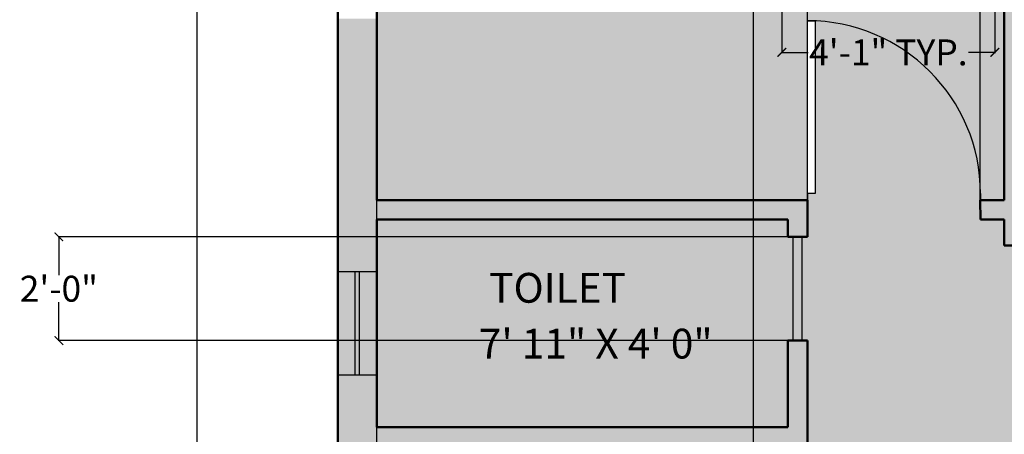
# Model space of a CAD drawing. Units: inches. Extents: x 528 to 2620, y -1066 to 798.
# Tile 25 of 41: x 983 to 1211, y 524 to 620. Entities that reach past the tile are written whole.
import ezdxf

# ---------------------------------------------------------------- set-up
doc = ezdxf.new("R2010")
doc.units = ezdxf.units.IN
doc.header["$MEASUREMENT"] = 0
for name, color, linetype, lineweight in [('A-ANNO-DIMS', 2, 'Continuous', 18), ('A-AREA-IDEN', 7, 'Continuous', 18), ('A-Door', 2, 'Continuous', 25), ('A-GLAZ', 3, 'Continuous', 25), ('A-WALL', 7, 'Continuous', 50), ('A-WALL-PATT', 8, 'Continuous', 13)]:
    doc.layers.add(name, color=color, linetype=linetype, lineweight=lineweight)
doc.styles.get("Standard").update_dxf_attribs({"font": 'arial.ttf'})
doc.dimstyles.get("Standard").update_dxf_attribs({"dimtxt": 6, "dimasz": 2, "dimexe": 0.18, "dimexo": 0.0625, "dimgap": 0.09, "dimtad": 0, "dimtih": 1, "dimtoh": 1, "dimdec": 1, "dimzin": 0, "dimdsep": 46, "dimlunit": 3, "dimtxsty": 'Standard', "dimblk": 'ARCHTICK', "dimcen": 0.09, "dimadec": 0, "dimazin": 0, "dimtfac": 1, "dimtdec": 1, "dimtofl": 0, "dimtmove": 0, "dimatfit": 3, "dimfxl": 1, "dimtolj": 1, "dimtzin": 0, "dimarcsym": 0})

# ---------------------------------------------------------------- blocks, each defined once
blk = doc.blocks.new('*U4')
for p, q in [((0, 0), (0, -6)), ((40, 0), (40, -6))]:
    blk.add_line(p, q)
blk.add_lwpolyline([(0, 0), (0, 40), (1.75, 40), (1.75, 0)], close=True)
blk.add_arc((0, 0), 40, 0, 90)
blk = doc.blocks.new('WIN-600')
for p, q in [((790.56, 714.92), (814.56, 714.92)), ((790.56, 713.92), (814.56, 713.92))]:
    blk.add_line(p, q)
blk.add_lwpolyline([(790.56, 718.92), (814.56, 718.92), (814.56, 709.92), (790.56, 709.92)], close=True)
blk = doc.blocks.new('_ArchTick')
at = {"color": 0, "linetype": 'ByBlock', "const_width": 0.15}
blk.add_lwpolyline([(-0.5, -0.5), (0.5, 0.5)], dxfattribs=at)
blk = doc.blocks.new('*D43')
at = {"layer": 'A-ANNO-DIMS', "color": 0, "lineweight": -2, "transparency": 16777216}
for p, q in [((1159.58, 623.98), (1159.58, 611.92)), ((1208.81, 623.98), (1208.81, 611.92)), ((1159.58, 612.1), (1165.7, 612.1)), ((1208.81, 612.1), (1202.7, 612.1))]:
    blk.add_line(p, q, dxfattribs=at)
at = {"layer": 'Defpoints', "color": 0, "transparency": 16777216}
for p in [(1159.58, 624.04), (1208.81, 624.04), (1208.81, 612.1)]:
    blk.add_point(p, dxfattribs=at)
at = {"layer": 'A-ANNO-DIMS', "color": 0, "lineweight": -2, "transparency": 16777216, "xscale": 2, "yscale": 2, "zscale": 2, "rotation": 180}
blk.add_blockref('_ArchTick', (1159.58, 612.1), dxfattribs=at)
at = {"layer": 'A-ANNO-DIMS', "color": 0, "lineweight": -2, "transparency": 16777216, "xscale": 2, "yscale": 2, "zscale": 2}
blk.add_blockref('_ArchTick', (1208.81, 612.1), dxfattribs=at)
at = {"layer": 'A-ANNO-DIMS', "color": 0, "transparency": 16777216, "insert": (1184.2, 612.1), "char_height": 6, "attachment_point": 5}
blk.add_mtext('\\A1;4\'-1" TYP.', dxfattribs=at)
blk = doc.blocks.new('*D58')
at = {"layer": 'A-ANNO-DIMS', "color": 0, "lineweight": -2, "transparency": 16777216}
for p, q in [((1165.5, 577.98), (1165.5, 751.1)), ((1165.5, 750.92), (1177.39, 750.92)), ((1205.42, 750.92), (1193.52, 750.92)), ((1205.42, 577.98), (1205.42, 751.1))]:
    blk.add_line(p, q, dxfattribs=at)
at = {"layer": 'Defpoints', "color": 0, "transparency": 16777216}
for p in [(1205.42, 750.92), (1165.5, 577.92), (1205.42, 577.92)]:
    blk.add_point(p, dxfattribs=at)
at = {"layer": 'A-ANNO-DIMS', "color": 0, "lineweight": -2, "transparency": 16777216, "xscale": 2, "yscale": 2, "zscale": 2, "rotation": 180}
blk.add_blockref('_ArchTick', (1165.5, 750.92), dxfattribs=at)
at = {"layer": 'A-ANNO-DIMS', "color": 0, "lineweight": -2, "transparency": 16777216, "xscale": 2, "yscale": 2, "zscale": 2}
blk.add_blockref('_ArchTick', (1205.42, 750.92), dxfattribs=at)
at = {"layer": 'A-ANNO-DIMS', "color": 0, "transparency": 16777216, "insert": (1185.46, 750.92), "char_height": 6, "attachment_point": 5}
blk.add_mtext('\\A1;3\'-4"', dxfattribs=at)
blk = doc.blocks.new('*D59')
at = {"layer": 'A-ANNO-DIMS', "color": 0, "lineweight": -2, "transparency": 16777216}
for p, q in [((1160.93, 569.42), (992.32, 569.42)), ((992.5, 569.42), (992.5, 560.58)), ((992.5, 545.42), (992.5, 554.27)), ((1160.93, 545.42), (992.32, 545.42))]:
    blk.add_line(p, q, dxfattribs=at)
at = {"layer": 'Defpoints', "color": 0, "transparency": 16777216}
for p in [(1161, 569.42), (992.5, 545.42), (1161, 545.42)]:
    blk.add_point(p, dxfattribs=at)
at = {"layer": 'A-ANNO-DIMS', "color": 0, "lineweight": -2, "transparency": 16777216, "xscale": 2, "yscale": 2, "zscale": 2}
for p, rotation in [((992.5, 569.42), 90), ((992.5, 545.42), 270)]:
    blk.add_blockref('_ArchTick', p, dxfattribs=dict(at, rotation=rotation))
at = {"layer": 'A-ANNO-DIMS', "color": 0, "transparency": 16777216, "insert": (992.5, 557.42), "char_height": 6, "attachment_point": 5}
blk.add_mtext('\\A1;2\'-0"', dxfattribs=at)
blk = doc.blocks.new('*D63')
at = {"layer": 'A-ANNO-DIMS', "color": 0, "lineweight": -2, "transparency": 16777216}
for p, q in [((1024.5, 405.4), (1024.5, 751.1)), ((1024.5, 750.92), (1025.64, 750.92)), ((1057, 750.92), (1055.85, 750.92)), ((1057, 405.4), (1057, 751.1))]:
    blk.add_line(p, q, dxfattribs=at)
at = {"layer": 'Defpoints', "color": 0, "transparency": 16777216}
for p in [(1057, 750.92), (1024.5, 405.34), (1057, 405.34)]:
    blk.add_point(p, dxfattribs=at)
at = {"layer": 'A-ANNO-DIMS', "color": 0, "lineweight": -2, "transparency": 16777216, "xscale": 2, "yscale": 2, "zscale": 2, "rotation": 180}
blk.add_blockref('_ArchTick', (1024.5, 750.92), dxfattribs=at)
at = {"layer": 'A-ANNO-DIMS', "color": 0, "lineweight": -2, "transparency": 16777216, "xscale": 2, "yscale": 2, "zscale": 2}
blk.add_blockref('_ArchTick', (1057, 750.92), dxfattribs=at)
at = {"layer": 'A-ANNO-DIMS', "color": 0, "transparency": 16777216, "insert": (1040.75, 750.92), "char_height": 6, "attachment_point": 5}
blk.add_mtext('\\A1;2\'-8 1/2"', dxfattribs=at)
blk = doc.blocks.new('*D66')
at = {"layer": 'A-ANNO-DIMS', "color": 0, "lineweight": -2, "transparency": 16777216}
for p, q in [((1066, 400.48), (1066, 751.1)), ((1066, 750.92), (1101.46, 750.92)), ((1153, 750.92), (1117.54, 750.92)), ((1153, 400.48), (1153, 751.1))]:
    blk.add_line(p, q, dxfattribs=at)
at = {"layer": 'Defpoints', "color": 0, "transparency": 16777216}
for p in [(1153, 750.92), (1066, 400.42), (1153, 400.42)]:
    blk.add_point(p, dxfattribs=at)
at = {"layer": 'A-ANNO-DIMS', "color": 0, "lineweight": -2, "transparency": 16777216, "xscale": 2, "yscale": 2, "zscale": 2, "rotation": 180}
blk.add_blockref('_ArchTick', (1066, 750.92), dxfattribs=at)
at = {"layer": 'A-ANNO-DIMS', "color": 0, "lineweight": -2, "transparency": 16777216, "xscale": 2, "yscale": 2, "zscale": 2}
blk.add_blockref('_ArchTick', (1153, 750.92), dxfattribs=at)
at = {"layer": 'A-ANNO-DIMS', "color": 0, "transparency": 16777216, "insert": (1109.5, 750.92), "char_height": 6, "attachment_point": 5}
blk.add_mtext('\\A1;7\'-3"', dxfattribs=at)

msp = doc.modelspace()

# ---------------------------------------------------------------- hatches: boundary and pattern name
at = {"layer": 'A-Door', "transparency": 33554521}
h = msp.add_hatch(color=256, dxfattribs=at)
h.dxf.hatch_style = 1
h.paths.add_polyline_path([(1164.19, 569.42), (1162.19, 569.42), (1162.19, 545.42), (1164.19, 545.42)])
at = {"layer": 'A-WALL-PATT', "transparency": 33554521}
h = msp.add_hatch(color=256, dxfattribs=at)
h.dxf.hatch_style = 1
h.paths.add_polyline_path([(1066, 709.92), (1114.5, 709.92), (1114.5, 718.92), (1057, 718.92), (1057, 667.92), (1066, 667.92)])
h.paths.add_polyline_path([(1227.5, 718.92), (1162.5, 718.92), (1162.5, 709.92), (1211, 709.92), (1211, 577.92), (1205.42, 577.92), (1205.5, 573.42), (1211, 573.42), (1211, 567.42), (1215.5, 567.42), (1215.5, 669.42), (1268, 669.42), (1268, 675.92), (1263.5, 675.92), (1263.5, 673.92), (1215.5, 673.92), (1215.5, 709.92), (1227.5, 709.92)])
h.paths.add_polyline_path([(1345, 718.92), (1316, 718.92), (1316, 709.92), (1336, 709.92), (1336, 641.67), (1345, 641.67)])
h.paths.add_polyline_path([(1066, 619.92), (1057, 619.92), (1057, 561.42), (1066, 561.42), (1066, 573.42), (1161, 573.42), (1161, 569.42), (1165.5, 569.42), (1165.5, 577.92), (1066, 577.92)])
h.paths.add_polyline_path([(1216, 391.42), (1216, 400.42), (1207, 400.42), (1201, 400.42), (1201, 397.42), (1201, 391.42), (1207, 391.42), (1207, 268.92), (1252, 268.92), (1252, 277.92), (1216, 277.92), (1216, 359.77)])
h.paths.add_polyline_path([(1345, 395.92), (1336, 395.92), (1288, 395.92), (1288, 391.42), (1336, 391.42), (1336, 277.92), (1300, 277.92), (1300, 268.92), (1345, 268.92)])
h.paths.add_polyline_path([(1345, 593.67), (1336, 593.67), (1336, 525.42), (1215.5, 525.42), (1215.5, 527.17), (1211, 527.17), (1211, 520.92), (1336, 520.92), (1336, 443.92), (1345, 443.92)])
h.paths.add_polyline_path([(1066, 520.92), (1165.5, 520.92), (1165.5, 545.42), (1161, 545.42), (1161, 525.42), (1066, 525.42), (1066, 537.42), (1057, 537.42), (1057, 484.67), (1066, 484.67)])
h.paths.add_polyline_path([(1066, 436.67), (1057, 436.67), (1057, 391.42), (1085.5, 391.42), (1085.5, 400.42), (1066, 400.42)])
h.paths.add_polyline_path([(1153, 397.42), (1153, 400.42), (1133.5, 400.42), (1133.5, 391.42), (1153, 391.42)])
at = {"layer": 'A-WALL-PATT', "transparency": 33554681}
h = msp.add_hatch(color=256, dxfattribs=at)
h.dxf.hatch_style = 1
h.paths.add_polyline_path([(1066, 665.92), (1062, 665.92), (1062, 621.92), (1066, 621.92)])
h.paths.add_polyline_path([(1061, 665.92), (1057, 665.92), (1057, 621.92), (1061, 621.92)])
h.paths.add_polyline_path([(1160.5, 713.92), (1116.5, 713.92), (1116.5, 709.92), (1160.5, 709.92)])
h.paths.add_polyline_path([(1160.5, 718.92), (1116.5, 718.92), (1116.5, 714.92), (1160.5, 714.92)])
h.paths.add_polyline_path([(1251.5, 713.92), (1227.5, 713.92), (1227.5, 709.92), (1251.5, 709.92)])
h.paths.add_polyline_path([(1251.5, 718.92), (1227.5, 718.92), (1227.5, 714.92), (1251.5, 714.92)])
h.paths.add_polyline_path([(1314, 713.92), (1270, 713.92), (1270, 709.92), (1314, 709.92)])
h.paths.add_polyline_path([(1314, 718.92), (1270, 718.92), (1270, 714.92), (1314, 714.92)])
h.paths.add_polyline_path([(1345, 639.67), (1341, 639.67), (1341, 595.67), (1345, 595.67)])
h.paths.add_polyline_path([(1340, 639.67), (1336, 639.67), (1336, 595.67), (1340, 595.67)])
h.paths.add_polyline_path([(1345, 441.92), (1341, 441.92), (1341, 397.92), (1345, 397.92)])
h.paths.add_polyline_path([(1340, 441.92), (1336, 441.92), (1336, 397.92), (1340, 397.92)])
h.paths.add_polyline_path([(1298, 272.92), (1254, 272.92), (1254, 268.92), (1298, 268.92)])
h.paths.add_polyline_path([(1298, 277.92), (1254, 277.92), (1254, 273.92), (1298, 273.92)])
h.paths.add_polyline_path([(1131.5, 395.42), (1087.5, 395.42), (1087.5, 391.42), (1131.5, 391.42)])
h.paths.add_polyline_path([(1131.5, 400.42), (1087.5, 400.42), (1087.5, 396.42), (1131.5, 396.42)])
h.paths.add_polyline_path([(1066, 482.67), (1062, 482.67), (1062, 438.67), (1066, 438.67)])
h.paths.add_polyline_path([(1061, 482.67), (1057, 482.67), (1057, 438.67), (1061, 438.67)])
h.paths.add_polyline_path([(1066, 561.42), (1062, 561.42), (1062, 537.42), (1066, 537.42)])
h.paths.add_polyline_path([(1061, 561.42), (1057, 561.42), (1057, 537.42), (1061, 537.42)])
at = {"layer": 'A-WALL-PATT', "transparency": 33554536}
h = msp.add_hatch(color=256, dxfattribs=at)
h.dxf.hatch_style = 1
h.paths.add_polyline_path([(1336, 709.92), (1268, 709.92), (1268, 699.92), (1266.75, 699.92), (1266.75, 675.92), (1268, 675.92), (1268, 669.42), (1215.5, 669.42), (1215.5, 567.17), (1217, 567.17), (1257, 567.17), (1257, 565.42), (1256.96, 565.42, -0.401453), (1217, 527.17), (1215.5, 527.17), (1215.5, 525.42), (1336, 525.42)], flags=17)
h.paths.add_polyline_path([(1285.03, 635.93), (1285.23, 636.13), (1285.67, 636.26), (1286.21, 636.02), (1286.98, 636.08), (1332.98, 636.08), (1333.36, 636.22), (1333.82, 636.08), (1334.11, 635.71), (1334.11, 635.3), (1333.91, 634.86), (1333.82, 634.83), (1333.82, 592.74), (1333.97, 592.6), (1334.11, 592.29), (1334.11, 591.88), (1333.82, 591.51), (1333.36, 591.37), (1332.98, 591.51), (1332.64, 591.79), (1332.64, 591.51), (1286.98, 591.51), (1286.17, 591.67), (1286.07, 591.57), (1285.68, 591.37), (1285.23, 591.51), (1285.03, 591.71), (1284.83, 592.1), (1284.98, 592.54), (1285.13, 592.69), (1285.13, 634.95), (1284.98, 635.1), (1284.83, 635.54)], flags=16)
h.paths.add_polyline_path([(1285.03, 635.93), (1285.23, 636.13), (1285.67, 636.26), (1286.21, 636.02), (1286.98, 636.08), (1332.98, 636.08), (1333.36, 636.22), (1333.82, 636.08), (1334.11, 635.71), (1334.11, 635.3), (1333.97, 634.99), (1333.82, 634.85), (1333.82, 592.74), (1333.97, 592.6), (1334.11, 592.29), (1334.11, 591.88), (1333.82, 591.51), (1333.36, 591.37), (1332.98, 591.51), (1332.64, 591.79), (1332.64, 592.25), (1332.64, 635.35), (1332.64, 635.8), (1332.98, 636.08), (1312.23, 636.08), (1311.1, 635.48), (1310.63, 635.48), (1310.43, 635.23), (1309.94, 635.1), (1309.7, 634.99), (1309.06, 634.76), (1308.71, 634.61), (1308.32, 634.61), (1307.75, 634.36), (1307.11, 634.27), (1307.01, 634.11), (1306.77, 634.02), (1307.25, 633.28), (1306.87, 633.04), (1306.77, 632.88), (1306.37, 632.64), (1306.03, 632.55), (1305.54, 632.41), (1315.47, 618.49), (1316.32, 619.39), (1312.77, 622.86), (1319.62, 630.11), (1320.07, 629.68), (1320.11, 630), (1320.28, 630.6), (1320.53, 631.18), (1320.53, 632.01), (1320.26, 632.55), (1320.11, 633.13), (1320.06, 633.73), (1320.63, 634.02), (1321.22, 634.16), (1321.86, 634.11), (1322.45, 633.91), (1322.99, 633.62), (1324.1, 633.62), (1324.64, 633.91), (1325.23, 634.07), (1325.87, 634.07), (1326.43, 633.91), (1326.98, 633.62), (1328.35, 633.62), (1328.9, 633.91), (1329.49, 634.11), (1330.1, 634.16), (1330.69, 634.02), (1331.28, 633.73), (1331.23, 633.13), (1331.09, 632.55), (1330.79, 632.01), (1330.79, 631.18), (1331.04, 630.6), (1331.23, 630), (1331.28, 629.41), (1331.19, 628.79), (1331.04, 628.18), (1330.79, 627.6), (1330.79, 626.77), (1331.04, 626.19), (1331.23, 625.59), (1331.28, 625.01), (1331.19, 624.38), (1331.04, 623.78), (1330.79, 623.24), (1330.79, 622.37), (1331.04, 621.83), (1331.23, 621.25), (1331.28, 620.6), (1331.19, 619.97), (1331.04, 619.37), (1330.79, 618.83), (1330.79, 617.96), (1331.09, 617.42), (1331.23, 616.88), (1331.28, 616.23), (1331.28, 615.52), (1330.69, 615.27), (1330.1, 615.12), (1329.49, 615.12), (1328.9, 615.32), (1328.35, 615.65), (1326.98, 615.65), (1326.43, 615.32), (1325.87, 615.16), (1325.23, 615.16), (1324.64, 615.32), (1324.1, 615.65), (1323.24, 615.65), (1324.93, 614.04), (1322.98, 611.98), (1324.1, 611.98), (1324.64, 612.27), (1325.28, 612.43), (1325.87, 612.43), (1326.48, 612.27), (1327.03, 611.98), (1328.35, 611.98), (1328.9, 612.27), (1329.49, 612.48), (1330.1, 612.52), (1330.74, 612.39), (1331.28, 612.07), (1331.28, 611.36), (1331.28, 610.75), (1331.09, 610.17), (1330.79, 609.63), (1330.79, 608.81), (1331.09, 608.22), (1331.23, 607.62), (1331.28, 606.99), (1331.23, 606.41), (1331.09, 605.81), (1330.79, 605.22), (1330.79, 604.4), (1331.09, 603.81), (1331.23, 603.21), (1331.28, 602.63), (1331.23, 602), (1331.09, 601.4), (1330.79, 600.86), (1330.79, 599.99), (1331.09, 599.45), (1331.23, 598.87), (1331.28, 598.22), (1331.23, 597.59), (1331.09, 596.99), (1330.79, 596.45), (1330.79, 595.58), (1331.09, 595.04), (1331.28, 594.51), (1331.28, 593.86), (1330.74, 593.61), (1330.1, 593.48), (1329.49, 593.48), (1328.9, 593.68), (1328.35, 594.01), (1327.03, 594.01), (1326.48, 593.68), (1325.87, 593.52), (1325.28, 593.52), (1324.64, 593.68), (1324.1, 594.01), (1323.04, 594.01), (1322.5, 593.68), (1321.91, 593.48), (1321.27, 593.48), (1320.63, 593.61), (1320.11, 593.86), (1320.11, 594.51), (1320.28, 595.04), (1320.58, 595.58), (1320.58, 596.45), (1320.28, 596.99), (1320.16, 597.59), (1320.1, 598.01), (1319.62, 597.55), (1315.66, 601.73), (1312.23, 591.57), (1311.74, 591.66), (1311.59, 591.91), (1310.78, 592.4), (1309.55, 592.89), (1308.96, 592.89), (1308.71, 593.03), (1308.56, 593.14), (1307.75, 593.52), (1306.77, 593.61), (1307.25, 594.36), (1306.87, 594.6), (1306.37, 594.84), (1306.03, 595.09), (1305.54, 595.24), (1315.46, 609.35), (1310.93, 613.71), (1315.47, 618.49), (1305.54, 632.41), (1306.03, 632.55), (1306.37, 632.64), (1306.77, 632.88), (1306.87, 633.04), (1307.25, 633.28), (1306.77, 634.02), (1307.01, 634.11), (1307.11, 634.27), (1307.75, 634.36), (1308.32, 634.61), (1308.71, 634.61), (1309.06, 634.76), (1309.7, 634.99), (1309.94, 635.1), (1310.43, 635.23), (1310.63, 635.48), (1311.1, 635.48), (1312.23, 636.08), (1286.98, 636.08), (1286.22, 636.02), (1286.41, 635.44), (1286.21, 635.05), (1286.02, 634.85), (1285.87, 634.81), (1285.87, 592.84), (1286.15, 592.73), (1286.41, 592.19), (1286.23, 591.66), (1286.17, 591.67), (1286.07, 591.57), (1285.68, 591.37), (1285.23, 591.51), (1285.03, 591.71), (1284.83, 592.1), (1284.98, 592.54), (1285.13, 592.69), (1285.13, 634.95), (1284.98, 635.1), (1284.83, 635.54)], flags=0)
h.paths.add_polyline_path([(1322.5, 653.6), (1333.65, 653.6), (1333.65, 637.99), (1322.5, 637.99)], flags=16)
h.paths.add_polyline_path([(1323.62, 652.48), (1332.53, 652.48), (1332.53, 639.11), (1323.62, 639.11)], flags=0)
edge = h.paths.add_edge_path(flags=0)
edge.add_ellipse((1328.07, 645.79), major_axis=(2.24, 2.24), ratio=1, start_angle=405, end_angle=495, ccw=False)
edge.add_ellipse((1328.07, 645.79), major_axis=(2.24, 2.24), ratio=1, start_angle=675, end_angle=765, ccw=False)
edge.add_ellipse((1328.07, 645.79), major_axis=(2.24, 2.24), ratio=1, start_angle=585, end_angle=675, ccw=False)
edge.add_ellipse((1328.07, 645.79), major_axis=(2.24, 2.24), ratio=1, start_angle=495, end_angle=585, ccw=False)
h.paths.add_polyline_path([(1320.58, 628.39), (1320.33, 628.01), (1320.61, 628.55)], flags=0)
h.paths.add_polyline_path([(1317.89, 604.89), (1318.78, 604.64), (1319.76, 604.28), (1318.88, 604.53)], flags=0)
h.paths.add_polyline_path([(1320.33, 599.65), (1320.58, 599.25), (1320.58, 599.16)], flags=0)
h.paths.add_polyline_path([(1322.5, 589.6), (1333.65, 589.6), (1333.65, 573.99), (1322.5, 573.99)], flags=16)
h.paths.add_polyline_path([(1323.62, 588.48), (1332.53, 588.48), (1332.53, 575.11), (1323.62, 575.11)], flags=0)
edge = h.paths.add_edge_path(flags=0)
edge.add_ellipse((1328.07, 581.8), major_axis=(-2.24, 2.24), ratio=1, start_angle=-45, end_angle=45, ccw=False)
edge.add_ellipse((1328.07, 581.8), major_axis=(-2.24, 2.24), ratio=1, start_angle=-135, end_angle=-45, ccw=False)
edge.add_ellipse((1328.07, 581.8), major_axis=(-2.24, 2.24), ratio=1, start_angle=135, end_angle=-135, ccw=False)
edge.add_ellipse((1328.07, 581.8), major_axis=(-2.24, 2.24), ratio=1, start_angle=45, end_angle=135, ccw=False)
h.paths.add_polyline_path([(1264.75, 699.92), (1263.5, 699.92), (1263.5, 709.92), (1215.5, 709.92), (1215.5, 673.92), (1263.5, 673.92), (1263.5, 675.92), (1264.75, 675.92)], flags=16)
h.paths.add_polyline_path([(1162.19, 569.42), (1161, 569.42), (1161, 573.42), (1066, 573.42), (1066, 525.42), (1161, 525.42), (1161, 545.42), (1162.19, 545.42)])
h.paths.add_polyline_path([(1256.96, 565.42), (1257, 565.42), (1257, 567.17), (1217, 567.17), (1215.5, 567.17), (1215.5, 567.42), (1211, 567.42), (1211, 573.42), (1205.5, 573.42), (1205.42, 577.92), (1211, 577.92), (1211, 709.92), (1066, 709.92), (1066, 577.92), (1165.5, 577.92), (1165.5, 569.42), (1164.19, 569.42), (1164.19, 545.42), (1165.5, 545.42), (1165.5, 520.92), (1153, 520.92), (1153, 484.92), (1102, 484.92), (1102, 436.42), (1153, 436.42), (1153, 400.42), (1153, 391.42), (1201, 391.42), (1201, 400.42), (1207, 400.42), (1216, 400.42), (1216, 391.42), (1216, 277.92), (1336, 277.92), (1336, 391.42), (1288, 391.42), (1288, 395.92), (1336, 395.92), (1336, 443.92), (1336, 520.92), (1211, 520.92), (1211, 527.17), (1215.5, 527.17), (1217, 527.17, 0.401453)])
h.paths.add_polyline_path([(1167.25, 579.42), (1165.5, 579.42), (1165.5, 619.42), (1167.25, 619.42)], flags=16)
h.paths.add_polyline_path([(1227.97, 501.56), (1236.36, 502.03), (1236.36, 492.55), (1227.97, 493.02, -0.254069)], flags=16)
h.paths.add_polyline_path([(1243.34, 515.69, -0.254069), (1251.88, 515.69), (1252.35, 507.3), (1242.87, 507.3)], flags=16)
h.paths.add_polyline_path([(1239.18, 504.68), (1256.03, 504.68), (1256.03, 479.42), (1239.18, 479.42)], flags=16)
h.paths.add_polyline_path([(1227.97, 489.6), (1236.36, 490.07), (1236.36, 480.59), (1227.97, 481.06, -0.254069)], flags=16)
h.paths.add_polyline_path([(1197.2, 624.04), (1197.2, 639.64), (1208.35, 639.64), (1208.35, 624.04)], flags=16)
h.paths.add_polyline_path([(1198.32, 625.15), (1198.32, 638.53), (1207.23, 638.53), (1207.23, 625.15)], flags=0)
h.paths.add_polyline_path([(1258.85, 502.03), (1267.25, 501.56, -0.254069), (1267.25, 493.02), (1258.85, 492.55)], flags=16)
h.paths.add_polyline_path([(1271.59, 519.66), (1333.67, 519.66), (1333.67, 451.59), (1319.09, 451.59), (1319.09, 505.07), (1288.09, 505.07), (1284.45, 505.07, -0.883215), (1270.68, 514.19), (1270.68, 518.75, -0.414214)], flags=16)
h.paths.add_polyline_path([(1331.85, 517.83), (1331.85, 453.42), (1328.2, 453.42), (1328.2, 505.07), (1298.42, 505.07), (1298.42, 514.19), (1288.09, 514.19), (1288.09, 517.83)], flags=0)
h.paths.add_polyline_path([(1242.87, 476.8), (1252.35, 476.8), (1251.88, 468.41, -0.254069), (1243.34, 468.41)], flags=16)
h.paths.add_polyline_path([(1258.85, 490.07), (1267.25, 489.6, -0.254069), (1267.25, 481.06), (1258.85, 480.59)], flags=16)
h.paths.add_polyline_path([(1161.68, 641.55), (1160.87, 641.72), (1160.77, 641.62), (1160.38, 641.41), (1159.93, 641.55), (1159.73, 641.75), (1159.53, 642.14), (1159.68, 642.58), (1159.83, 642.73), (1159.83, 684.99), (1159.68, 685.14), (1159.53, 685.58), (1159.73, 685.97), (1159.93, 686.17), (1160.37, 686.31), (1160.91, 686.06), (1161.68, 686.13), (1207.68, 686.13), (1208.06, 686.27), (1208.52, 686.13), (1208.81, 685.76), (1208.81, 685.34), (1208.61, 684.9), (1208.52, 684.87), (1208.52, 642.78), (1208.67, 642.65), (1208.88, 642.2), (1208.72, 641.8), (1208.52, 641.55), (1208.06, 641.41), (1207.68, 641.55), (1207.34, 641.83), (1207.34, 641.55)], flags=16)
h.paths.add_polyline_path([(1186.93, 641.62), (1186.44, 641.71), (1186.29, 641.95), (1185.48, 642.45), (1184.25, 642.94), (1183.66, 642.94), (1183.41, 643.07), (1183.26, 643.18), (1182.45, 643.57), (1181.47, 643.65), (1181.95, 644.4), (1181.57, 644.64), (1181.07, 644.89), (1180.73, 645.13), (1180.24, 645.29), (1190.16, 659.4), (1185.63, 663.75), (1190.17, 668.54), (1180.24, 682.46), (1180.73, 682.59), (1181.07, 682.68), (1181.47, 682.93), (1181.57, 683.08), (1181.95, 683.33), (1181.47, 684.07), (1181.71, 684.16), (1181.81, 684.31), (1182.45, 684.4), (1183.02, 684.65), (1183.41, 684.65), (1183.76, 684.81), (1184.4, 685.03), (1184.64, 685.14), (1185.13, 685.28), (1185.33, 685.52), (1185.8, 685.52), (1186.93, 686.13), (1161.68, 686.13), (1160.92, 686.06), (1161.11, 685.49), (1160.91, 685.1), (1160.72, 684.9), (1160.57, 684.85), (1160.57, 642.88), (1160.85, 642.77), (1161.11, 642.23), (1160.93, 641.7), (1160.87, 641.72), (1160.77, 641.62), (1160.38, 641.41), (1159.93, 641.55), (1159.73, 641.75), (1159.53, 642.14), (1159.68, 642.58), (1159.83, 642.73), (1159.83, 684.99), (1159.68, 685.14), (1159.53, 685.58), (1159.73, 685.97), (1159.93, 686.17), (1160.37, 686.31), (1160.91, 686.06), (1161.68, 686.13), (1207.68, 686.13), (1208.06, 686.27), (1208.52, 686.13), (1208.81, 685.76), (1208.81, 685.34), (1208.67, 685.03), (1208.52, 684.9), (1208.52, 642.78), (1208.67, 642.65), (1208.88, 642.2), (1208.72, 641.8), (1208.52, 641.55), (1208.06, 641.41), (1207.68, 641.55), (1207.34, 641.83), (1207.34, 642.29), (1207.34, 685.39), (1207.34, 685.85), (1207.68, 686.13), (1186.93, 686.13), (1185.8, 685.52), (1185.33, 685.52), (1185.13, 685.28), (1184.64, 685.14), (1184.4, 685.03), (1183.76, 684.81), (1183.41, 684.65), (1183.02, 684.65), (1182.45, 684.4), (1181.81, 684.31), (1181.71, 684.16), (1181.47, 684.07), (1181.95, 683.33), (1181.57, 683.08), (1181.47, 682.93), (1181.07, 682.68), (1180.73, 682.59), (1180.24, 682.46), (1190.17, 668.54), (1191.02, 669.43), (1187.47, 672.9), (1194.32, 680.15), (1194.77, 679.72), (1194.81, 680.04), (1194.98, 680.65), (1195.23, 681.23), (1195.23, 682.05), (1194.96, 682.59), (1194.81, 683.17), (1194.76, 683.78), (1195.33, 684.07), (1195.92, 684.2), (1196.56, 684.16), (1197.15, 683.96), (1197.69, 683.67), (1198.8, 683.67), (1199.34, 683.96), (1199.93, 684.11), (1200.57, 684.11), (1201.13, 683.96), (1201.68, 683.67), (1203.05, 683.67), (1203.6, 683.96), (1204.19, 684.16), (1204.8, 684.2), (1205.39, 684.07), (1205.98, 683.78), (1205.93, 683.17), (1205.79, 682.59), (1205.49, 682.05), (1205.49, 681.23), (1205.74, 680.65), (1205.93, 680.04), (1205.98, 679.46), (1205.89, 678.83), (1205.74, 678.23), (1205.49, 677.65), (1205.49, 676.82), (1205.74, 676.24), (1205.93, 675.63), (1205.98, 675.05), (1205.89, 674.42), (1205.74, 673.82), (1205.49, 673.28), (1205.49, 672.41), (1205.74, 671.87), (1205.93, 671.29), (1205.98, 670.64), (1205.89, 670.02), (1205.74, 669.41), (1205.49, 668.87), (1205.49, 668), (1205.79, 667.46), (1205.93, 666.93), (1205.98, 666.28), (1205.98, 665.56), (1205.39, 665.32), (1204.8, 665.16), (1204.19, 665.16), (1203.6, 665.36), (1203.05, 665.7), (1201.68, 665.7), (1201.13, 665.36), (1200.57, 665.2), (1199.93, 665.2), (1199.34, 665.36), (1198.8, 665.7), (1197.94, 665.7), (1199.63, 664.09), (1197.68, 662.03), (1198.8, 662.03), (1199.34, 662.32), (1199.98, 662.47), (1200.57, 662.47), (1201.18, 662.32), (1201.73, 662.03), (1203.05, 662.03), (1203.6, 662.32), (1204.19, 662.52), (1204.8, 662.56), (1205.44, 662.43), (1205.98, 662.12), (1205.98, 661.4), (1205.98, 660.8), (1205.79, 660.21), (1205.49, 659.68), (1205.49, 658.85), (1205.79, 658.27), (1205.93, 657.66), (1205.98, 657.04), (1205.93, 656.45), (1205.79, 655.85), (1205.49, 655.27), (1205.49, 654.44), (1205.79, 653.86), (1205.93, 653.25), (1205.98, 652.67), (1205.93, 652.05), (1205.79, 651.44), (1205.49, 650.91), (1205.49, 650.03), (1205.79, 649.5), (1205.93, 648.91), (1205.98, 648.26), (1205.93, 647.64), (1205.79, 647.03), (1205.49, 646.5), (1205.49, 645.62), (1205.79, 645.09), (1205.98, 644.55), (1205.98, 643.9), (1205.44, 643.65), (1204.8, 643.52), (1204.19, 643.52), (1203.6, 643.72), (1203.05, 644.06), (1201.73, 644.06), (1201.18, 643.72), (1200.57, 643.57), (1199.98, 643.57), (1199.34, 643.72), (1198.8, 644.06), (1197.74, 644.06), (1197.2, 643.72), (1196.61, 643.52), (1195.97, 643.52), (1195.33, 643.65), (1194.81, 643.9), (1194.81, 644.55), (1194.98, 645.09), (1195.28, 645.62), (1195.28, 646.5), (1194.98, 647.03), (1194.86, 647.64), (1194.8, 648.06), (1194.32, 647.59), (1190.36, 651.77)], flags=16)
h.paths.add_polyline_path([(1195.28, 649.2), (1195.03, 649.7), (1195.28, 649.29)], flags=0)
h.paths.add_polyline_path([(1194.46, 654.33), (1193.58, 654.58), (1192.59, 654.93), (1193.48, 654.69)], flags=0)
h.paths.add_polyline_path([(1195.28, 678.43), (1195.03, 678.05), (1195.31, 678.59)], flags=0)
h.paths.add_polyline_path([(1197.2, 688.04), (1197.2, 703.64), (1208.35, 703.64), (1208.35, 688.04)], flags=16)
h.paths.add_polyline_path([(1198.32, 689.15), (1198.32, 702.53), (1207.23, 702.53), (1207.23, 689.15)], flags=0)
h.paths.add_polyline_path([(1217.1, 329.02), (1230.65, 329.02), (1230.65, 315.47), (1217.1, 315.47)], flags=16)
h.paths.add_polyline_path([(1223.87, 322.24), (1227.26, 322.24), (1227.26, 321.32, -0.414214), (1229.73, 318.86, -1), (1224.8, 318.86), (1223.87, 318.86)], flags=0)
h.paths.add_polyline_path([(1222.11, 325.63, -1), (1218.86, 325.63, -1)], flags=0)
h.paths.add_polyline_path([(1228.25, 325.63, -1), (1226.28, 325.63, -1)], flags=0)
h.paths.add_polyline_path([(1221.53, 318.86, -1), (1219.44, 318.86, -1)], flags=0)
h.paths.add_polyline_path([(1299.15, 293.73), (1299.15, 278.54), (1271.23, 278.54), (1271.23, 293.73)], flags=16)
h.paths.add_polyline_path([(1259.69, 292.21), (1270.62, 292.21, -1), (1270.62, 291.6), (1259.69, 291.6, -1)], flags=16)
h.paths.add_polyline_path([(1259.69, 291.3), (1270.62, 291.3, -1), (1270.62, 290.69), (1259.69, 290.69, -1)], flags=16)
h.paths.add_polyline_path([(1259.69, 290.39), (1270.62, 290.39, -1), (1270.62, 289.78), (1259.69, 289.78, -1)], flags=16)
h.paths.add_polyline_path([(1259.69, 289.48), (1270.62, 289.48, -1), (1270.62, 288.87), (1259.69, 288.87, -1)], flags=16)
h.paths.add_polyline_path([(1259.69, 288.57), (1270.62, 288.57, -1), (1270.62, 287.96), (1259.69, 287.96, -1)], flags=16)
h.paths.add_polyline_path([(1274.41, 292.38), (1283.25, 292.38, -0.414214), (1285.07, 290.56), (1285.07, 283.64, -0.414214), (1283.25, 281.82), (1277.72, 281.82), (1278.67, 280.87, -0.57735), (1279.38, 280.16), (1279.44, 280.11, -1), (1279.03, 279.7), (1278.97, 279.75, -0.57735), (1278.26, 280.46), (1276.9, 281.82), (1274.41, 281.82, -0.414214), (1272.58, 283.64), (1272.58, 290.56, -0.414214)], flags=0)
h.paths.add_polyline_path([(1259.69, 287.65), (1270.62, 287.65, -1), (1270.62, 287.05), (1259.69, 287.05, -1)], flags=16)
h.paths.add_polyline_path([(1259.69, 286.74), (1270.62, 286.74, -1), (1270.62, 286.14), (1259.69, 286.14, -1)], flags=16)
h.paths.add_polyline_path([(1259.69, 285.83), (1270.62, 285.83, -1), (1270.62, 285.22), (1259.69, 285.22, -1)], flags=16)
h.paths.add_polyline_path([(1259.69, 284.92), (1270.62, 284.92, -1), (1270.62, 284.31), (1259.69, 284.31, -1)], flags=16)
h.paths.add_polyline_path([(1259.69, 284.01), (1270.62, 284.01, -1), (1270.62, 283.4), (1259.69, 283.4, -1)], flags=16)
h.paths.add_polyline_path([(1287.82, 292.38), (1296.67, 292.38, -0.414214), (1298.49, 290.56), (1298.49, 283.64, -0.414214), (1296.67, 281.82), (1291.14, 281.82), (1292.09, 280.87, -0.57735), (1292.8, 280.16), (1292.85, 280.11, -1), (1292.44, 279.7), (1292.39, 279.75, -0.57735), (1291.68, 280.46), (1290.32, 281.82), (1287.82, 281.82, -0.414214), (1286, 283.64), (1286, 290.56, -0.414214)], flags=0)
h.paths.add_polyline_path([(1259.69, 283.1), (1270.62, 283.1, -1), (1270.62, 282.49), (1259.69, 282.49, -1)], flags=16)
h.paths.add_polyline_path([(1279.94, 287.61, -1), (1278.01, 287.61, -1)], flags=0)
h.paths.add_polyline_path([(1259.69, 282.19), (1270.62, 282.19, -1), (1270.62, 281.58), (1259.69, 281.58, -1)], flags=16)
h.paths.add_polyline_path([(1259.69, 281.27), (1270.62, 281.27, -1), (1270.62, 280.67), (1259.69, 280.67, -1)], flags=16)
h.paths.add_polyline_path([(1275.16, 284.17, -1), (1274.77, 284.17, -1)], flags=0)
h.paths.add_polyline_path([(1293.36, 287.61, -1), (1291.43, 287.61, -1)], flags=0)
h.paths.add_polyline_path([(1275.14, 280.5), (1276.33, 280.5, -5.828427), (1276.33, 280.12), (1275.14, 280.12, -1)], flags=0)
h.paths.add_polyline_path([(1288.57, 284.17, -1), (1288.19, 284.17, -1)], flags=0)
h.paths.add_polyline_path([(1281.31, 280.5), (1282.5, 280.5, -1), (1282.5, 280.12), (1281.31, 280.12, -5.828427)], flags=0)
h.paths.add_polyline_path([(1288.56, 280.5), (1289.75, 280.5, -5.828427), (1289.75, 280.12), (1288.56, 280.12, -1)], flags=0)
h.paths.add_polyline_path([(1294.73, 280.5), (1295.92, 280.5, -1), (1295.92, 280.12), (1294.73, 280.12, -5.828427)], flags=0)
h.paths.add_polyline_path([(1207, 391.42), (1201, 391.42), (1061.5, 391.42), (1061.5, 307.96), (1069, 307.96), (1069, 305.42), (1207, 305.42)])
at = {"layer": 'A-WALL-PATT', "transparency": 33554480}
h = msp.add_hatch(color=256, dxfattribs=at)
h.dxf.hatch_style = 1
h.paths.add_polyline_path([(1211, 709.92), (1066, 709.92), (1066, 577.92), (1165.5, 577.92), (1165.5, 579.42), (1165.5, 619.42), (1167.25, 619.42), (1167.25, 619.38, -0.401453), (1205.5, 579.42), (1205.5, 577.92), (1211, 577.92)])
h.paths.add_polyline_path([(1160.83, 686.06), (1160.91, 686.06), (1160.77, 686.13)], flags=16)
h.paths.add_polyline_path([(1160.93, 641.7), (1160.93, 641.71), (1160.93, 641.7)], flags=0)
h.paths.add_polyline_path([(1159.83, 684.99), (1159.58, 685.24), (1159.58, 685.82), (1160.02, 686.26), (1160.22, 686.26), (1159.93, 686.17), (1159.73, 685.97), (1159.58, 685.68), (1159.58, 685.43), (1159.68, 685.14), (1159.88, 684.94), (1160.17, 684.81), (1160.42, 684.81), (1160.72, 684.9), (1160.91, 685.1), (1161.11, 685.49), (1161.06, 685.64), (1161.06, 685.25), (1160.57, 684.75), (1160.57, 642.96), (1161.06, 642.51), (1161.06, 641.89), (1160.87, 641.72), (1161.68, 641.55), (1186.53, 641.55), (1186.29, 641.95), (1185.48, 642.45), (1184.25, 642.94), (1183.59, 642.94), (1183.26, 643.18), (1182.45, 643.57), (1181.47, 643.65), (1181.95, 644.4), (1181.57, 644.64), (1181.07, 644.89), (1180.73, 645.13), (1180.24, 645.29), (1190.16, 659.4), (1185.63, 663.75), (1190.17, 668.54), (1180.24, 682.46), (1180.73, 682.59), (1181.07, 682.68), (1181.47, 682.93), (1181.57, 683.08), (1181.95, 683.33), (1181.47, 684.07), (1181.71, 684.16), (1181.81, 684.31), (1182.45, 684.4), (1183.02, 684.65), (1183.41, 684.65), (1183.76, 684.81), (1184.4, 685.03), (1184.64, 685.14), (1185.13, 685.28), (1185.33, 685.52), (1185.8, 685.52), (1186.93, 686.13), (1207.68, 686.13), (1208.06, 686.27), (1208.63, 686.09), (1208.88, 685.48), (1208.61, 684.9), (1208.52, 684.87), (1208.52, 642.78), (1208.81, 642.51), (1208.81, 641.92), (1208.45, 641.46), (1207.79, 641.46), (1207.34, 641.83), (1207.34, 641.55), (1161.68, 641.55), (1160.93, 641.7), (1160.38, 641.41), (1159.82, 641.59), (1159.53, 642.14), (1159.72, 642.7), (1159.83, 642.76)], flags=16)
h.paths.add_polyline_path([(1159.83, 684.99), (1159.58, 685.24), (1159.58, 685.82), (1160.02, 686.26), (1160.22, 686.26), (1159.93, 686.17), (1159.73, 685.97), (1159.58, 685.68), (1159.58, 685.43), (1159.68, 685.14), (1159.83, 684.99), (1159.83, 642.73), (1159.68, 642.58), (1159.58, 642.29), (1159.58, 642.04), (1159.73, 641.75), (1160.02, 641.46), (1160.22, 641.46), (1159.82, 641.59), (1159.53, 642.14), (1159.68, 642.58), (1159.83, 642.73)], flags=0)
h.paths.add_polyline_path([(1207.68, 686.13), (1207.52, 686.13), (1207.49, 686.06)], flags=0)
h.paths.add_polyline_path([(1195.28, 648.71), (1195.29, 648.52), (1195.52, 648.75), (1195.52, 648.8), (1195.28, 649.2)], flags=0)
h.paths.add_polyline_path([(1194.77, 679.72), (1194.81, 680.04), (1194.98, 680.65), (1195.23, 681.23), (1195.23, 682.05), (1194.96, 682.59), (1194.81, 683.17), (1194.76, 683.78), (1195.33, 684.07), (1195.92, 684.2), (1196.56, 684.16), (1197.15, 683.96), (1197.69, 683.67), (1198.8, 683.67), (1199.34, 683.96), (1199.93, 684.11), (1200.57, 684.11), (1201.13, 683.96), (1201.68, 683.67), (1203.05, 683.67), (1203.6, 683.96), (1204.19, 684.16), (1204.8, 684.2), (1205.39, 684.07), (1205.98, 683.78), (1205.93, 683.17), (1205.79, 682.59), (1205.49, 682.05), (1205.49, 681.23), (1205.74, 680.65), (1205.93, 680.04), (1205.98, 679.46), (1205.89, 678.83), (1205.74, 678.23), (1205.49, 677.65), (1205.49, 676.82), (1205.74, 676.24), (1205.93, 675.63), (1205.98, 675.05), (1205.89, 674.42), (1205.74, 673.82), (1205.49, 673.28), (1205.49, 672.41), (1205.74, 671.87), (1205.93, 671.29), (1205.98, 670.64), (1205.89, 670.02), (1205.74, 669.41), (1205.49, 668.87), (1205.49, 668), (1205.79, 667.46), (1205.93, 666.93), (1205.98, 666.28), (1205.98, 665.56), (1205.39, 665.32), (1204.8, 665.16), (1204.19, 665.16), (1203.6, 665.36), (1203.05, 665.7), (1201.68, 665.7), (1201.13, 665.36), (1200.57, 665.2), (1199.93, 665.2), (1199.34, 665.36), (1198.8, 665.7), (1197.94, 665.7), (1199.63, 664.09), (1197.68, 662.03), (1198.8, 662.03), (1199.34, 662.32), (1199.98, 662.47), (1200.57, 662.47), (1201.18, 662.32), (1201.73, 662.03), (1203.05, 662.03), (1203.6, 662.32), (1204.19, 662.52), (1204.8, 662.56), (1205.44, 662.43), (1205.98, 662.12), (1205.98, 661.4), (1205.98, 660.8), (1205.79, 660.21), (1205.49, 659.68), (1205.49, 658.85), (1205.79, 658.27), (1205.93, 657.66), (1205.98, 657.04), (1205.93, 656.45), (1205.79, 655.85), (1205.49, 655.27), (1205.49, 654.44), (1205.79, 653.86), (1205.93, 653.25), (1205.98, 652.67), (1205.93, 652.05), (1205.79, 651.44), (1205.49, 650.91), (1205.49, 650.03), (1205.79, 649.5), (1205.93, 648.91), (1205.98, 648.26), (1205.93, 647.64), (1205.79, 647.03), (1205.49, 646.5), (1205.49, 645.62), (1205.79, 645.09), (1205.98, 644.55), (1205.98, 643.9), (1205.44, 643.65), (1204.8, 643.52), (1204.19, 643.52), (1203.6, 643.72), (1203.05, 644.06), (1201.73, 644.06), (1201.18, 643.72), (1200.57, 643.57), (1199.98, 643.57), (1199.34, 643.72), (1198.8, 644.06), (1197.74, 644.06), (1195.52, 644.3), (1205.29, 644.3), (1205.29, 661.45), (1197.13, 661.45), (1199.63, 664.09), (1196, 667.54), (1201.48, 673.28), (1195.52, 679), (1195.52, 678.92), (1195.31, 678.58), (1195.28, 678.43), (1195.03, 678.05), (1195.28, 678.52), (1195.28, 679.23)], flags=0)
h.paths.add_polyline_path([(1192.59, 654.93), (1193.48, 654.69), (1194.46, 654.33), (1193.58, 654.58)], flags=0)
h.paths.add_polyline_path([(1192.59, 672.79), (1193.43, 673.04), (1194.3, 673.35), (1194.29, 673.36), (1193.58, 673.15)], flags=0)
h.paths.add_polyline_path([(1195.28, 649.29), (1195.03, 649.7), (1195.3, 649.17)], flags=0)
h.paths.add_polyline_path([(1197.2, 639.64), (1208.35, 639.64), (1208.35, 624.04), (1197.2, 624.04)], flags=16)
h.paths.add_polyline_path([(1198.32, 638.53), (1207.23, 638.53), (1207.23, 625.15), (1198.32, 625.15)], flags=0)
edge = h.paths.add_edge_path(flags=0)
edge.add_ellipse((1202.77, 631.84), major_axis=(-2.24, 2.24), ratio=1, start_angle=-45, end_angle=45, ccw=False)
edge.add_ellipse((1202.77, 631.84), major_axis=(-2.24, 2.24), ratio=1, start_angle=-135, end_angle=-45, ccw=False)
edge.add_ellipse((1202.77, 631.84), major_axis=(-2.24, 2.24), ratio=1, start_angle=135, end_angle=-135, ccw=False)
edge.add_ellipse((1202.77, 631.84), major_axis=(-2.24, 2.24), ratio=1, start_angle=45, end_angle=135, ccw=False)
h.paths.add_polyline_path([(1197.2, 688.04), (1197.2, 703.64), (1208.35, 703.64), (1208.35, 688.04)], flags=16)
h.paths.add_polyline_path([(1198.32, 689.15), (1198.32, 702.53), (1207.23, 702.53), (1207.23, 689.15)], flags=0)
edge = h.paths.add_edge_path(flags=0)
edge.add_ellipse((1202.77, 695.84), major_axis=(2.24, 2.24), ratio=1, start_angle=405, end_angle=495, ccw=False)
edge.add_ellipse((1202.77, 695.84), major_axis=(2.24, 2.24), ratio=1, start_angle=675, end_angle=765, ccw=False)
edge.add_ellipse((1202.77, 695.84), major_axis=(2.24, 2.24), ratio=1, start_angle=585, end_angle=675, ccw=False)
edge.add_ellipse((1202.77, 695.84), major_axis=(2.24, 2.24), ratio=1, start_angle=495, end_angle=585, ccw=False)
h.paths.add_polyline_path([(1207.34, 685.39), (1207.34, 685.85), (1207.79, 686.22), (1208.45, 686.22), (1208.81, 685.76), (1208.81, 685.17), (1208.52, 684.9), (1208.52, 642.78), (1208.81, 642.51), (1208.81, 641.92), (1208.45, 641.46), (1207.79, 641.46), (1207.34, 641.83), (1207.34, 642.29)], flags=0)
h.paths.add_polyline_path([(1207.47, 642.68), (1207.99, 643.01), (1208.61, 642.77), (1208.88, 642.2), (1208.63, 641.59), (1208.06, 641.41), (1207.49, 641.62), (1207.28, 642.13)], flags=16)
h.paths.add_polyline_path([(1207.63, 684.9), (1207.88, 684.74), (1208.35, 684.74), (1208.67, 685.03), (1208.81, 685.34), (1208.81, 685.64), (1208.72, 685.88), (1208.45, 686.22), (1208.22, 686.22), (1208.63, 686.09), (1208.88, 685.48), (1208.67, 685.03), (1208.35, 684.74), (1207.79, 684.74)], flags=16)
h.paths.add_polyline_path([(1076.48, 648.31), (1137.07, 648.31), (1137.07, 658.87), (1076.48, 658.87)], flags=24)
h.paths.add_polyline_path([(1076.71, 662.1), (1130.01, 662.1), (1130.01, 672.8), (1076.71, 672.8)], flags=24)
at = {"layer": 'A-WALL-PATT', "transparency": 33554536}
h = msp.add_hatch(color=256, dxfattribs=at)
h.dxf.hatch_style = 1
h.paths.add_polyline_path([(1340, 441.92), (1336, 441.92), (1336, 397.92), (1340, 397.92)])
h.paths.add_polyline_path([(1345, 443.92), (1336, 443.92), (1336, 441.92), (1340, 441.92), (1345, 441.92)])
h.paths.add_polyline_path([(1345, 397.92), (1336, 397.92), (1336, 395.92), (1345, 395.92)])
h.paths.add_polyline_path([(1341, 441.92), (1340, 441.92), (1340, 397.92), (1341, 397.92)])
h.paths.add_polyline_path([(1345, 595.67), (1336, 595.67), (1336, 593.67), (1345, 593.67)])
h.paths.add_polyline_path([(1345, 641.67), (1336, 641.67), (1336, 639.67), (1345, 639.67)])
h.paths.add_polyline_path([(1341, 639.67), (1340, 639.67), (1340, 595.67), (1341, 595.67)])
h.paths.add_polyline_path([(1062, 561.42), (1061, 561.42), (1061, 537.42), (1062, 537.42)])

# ---------------------------------------------------------------- linework, layer by layer
at = {"layer": 'A-Door'}
msp.add_lwpolyline([(1164.19, 545.42), (1162.19, 545.42), (1162.19, 569.42), (1164.19, 569.42)], close=True, dxfattribs=at)
at = {"layer": 'A-WALL'}
for p, q in [((1057, 718.92), (1057, 391.42)), ((1066, 709.92), (1066, 577.92)), ((1211, 709.92), (1211, 577.92)), ((1165.5, 577.92), (1066, 577.92)), ((1165.5, 577.92), (1165.5, 569.42)), ((1205.42, 577.92), (1211, 577.92)), ((1205.5, 573.42), (1205.42, 577.92)), ((1161, 573.42), (1066, 573.42)), ((1066, 573.42), (1066, 525.42)), ((1161, 573.42), (1161, 569.42)), ((1205.5, 573.42), (1211, 573.42)), ((1211, 573.42), (1211, 567.42)), ((1161, 569.42), (1165.5, 569.42)), ((1211, 567.42), (1215.5, 567.42)), ((1161, 545.42), (1161, 525.42)), ((1161, 545.42), (1165.5, 545.42)), ((1165.5, 545.42), (1165.5, 520.92)), ((1161, 525.42), (1066, 525.42))]:
    msp.add_line(p, q, dxfattribs=at)

# ---------------------------------------------------------------- block references
at = {"layer": 'A-Door'}
msp.add_blockref('*U4', (1165.5, 579.42), dxfattribs=at)
at = {"layer": 'A-GLAZ', "rotation": 89.99999999999925}
msp.add_blockref('WIN-600', (1775.92, -253.14), dxfattribs=at)

# ---------------------------------------------------------------- texts
at = {"layer": 'A-AREA-IDEN'}
for s, height, p in [('TOILET', 6.891, (1091.95, 554.18)), ('7\' 11" X 4\' 0"', 6.8907, (1089.56, 541.27))]:
    msp.add_text(s, height=height, dxfattribs=at).set_placement(p)

# ---------------------------------------------------------------- dimensions: what is measured, and where the dimension line sits
at = {"layer": 'A-ANNO-DIMS'}
for base, p1, p2, picture, middle in [((1057, 750.92), (1024.5, 405.34), (1057, 405.34), '*D63', (1040.75, 750.92)), ((1153, 750.92), (1066, 400.42), (1153, 400.42), '*D66', (1109.5, 750.92)), ((1205.42, 750.92), (1165.5, 577.92), (1205.42, 577.92), '*D58', (1185.46, 750.92))]:
    dim = msp.add_linear_dim(base=base, p1=p1, p2=p2, dimstyle='Standard', override={"dimdec": 1, "dimlfac": 1, "dimrnd": 0, "dimzin": 1, "dimdsep": 46, "dimlunit": 4, "dimfrac": 2}, dxfattribs=at)
    dim.commit()
    dim.dimension.update_dxf_attribs({"geometry": picture, "text_midpoint": middle})
dim = msp.add_linear_dim(base=(1208.81, 612.1), p1=(1159.58, 624.04), p2=(1208.81, 624.04), text='<> TYP.', dimstyle='Standard', override={"dimdec": 1, "dimrnd": 0, "dimzin": 1, "dimlunit": 4, "dimfrac": 2}, dxfattribs=at)
dim.commit()
dim.dimension.update_dxf_attribs({"geometry": '*D43', "text_midpoint": (1184.2, 612.1)})
dim = msp.add_linear_dim(base=(992.5, 545.42), p1=(1161, 569.42), p2=(1161, 545.42), angle=90, dimstyle='Standard', override={"dimdec": 1, "dimlfac": 1, "dimrnd": 0, "dimzin": 1, "dimdsep": 46, "dimlunit": 4, "dimfrac": 2}, dxfattribs=at)
dim.commit()
dim.dimension.update_dxf_attribs({"geometry": '*D59', "text_midpoint": (992.5, 557.42)})

doc.saveas('drawing.dxf')
